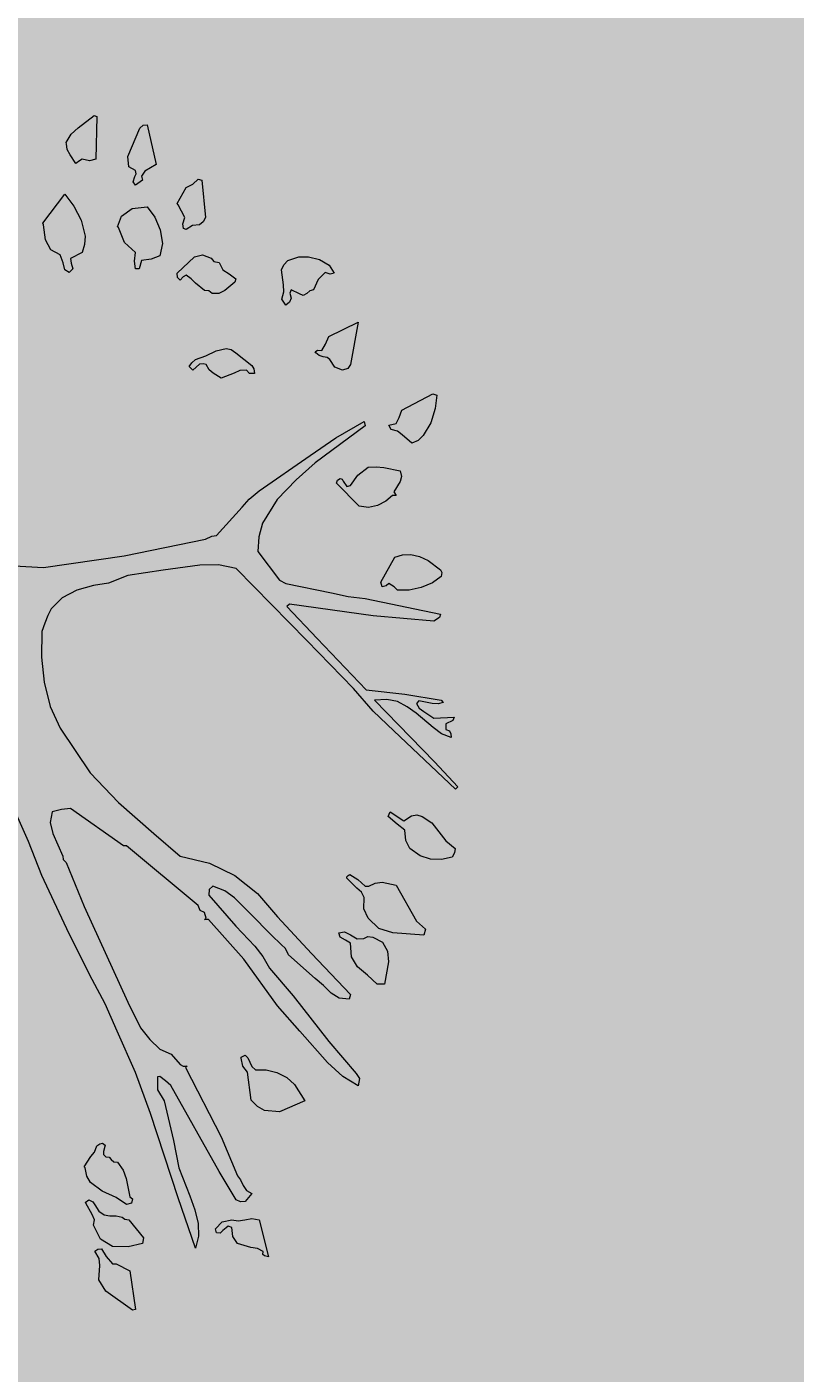
# Model space of a CAD drawing. Units: inches. Extents: x 84 to 1044, y -280 to 906.
# Tile 71 of 105: x 718.82 to 732.52, y 408.34 to 432.35. Entities that reach past the tile are written whole.
import ezdxf

# ---------------------------------------------------------------- set-up
doc = ezdxf.new("R2010")
doc.units = ezdxf.units.IN
doc.layers.add('A-ANNO-DIMS', color=2, linetype='Continuous', lineweight=18)
doc.layers.add('L-PLNT', color=114, linetype='Continuous', lineweight=15)
doc.layers.add('L-PLNT-PATT', color=9, linetype='Continuous', lineweight=9, true_color=0xafd9aa)
doc.styles.get("Standard").update_dxf_attribs({"font": 'arial.ttf'})
doc.dimstyles.get("Standard").update_dxf_attribs({"dimtxt": 0.18, "dimasz": 0.18, "dimexe": 0.18, "dimexo": 0.0625, "dimgap": 0.09, "dimtad": 0, "dimtih": 1, "dimtoh": 1, "dimdec": 4, "dimzin": 0, "dimdsep": 46, "dimtxsty": 'Standard', "dimcen": 0.09, "dimadec": 0, "dimazin": 0, "dimtfac": 1, "dimtdec": 4, "dimtofl": 0, "dimtmove": 0, "dimatfit": 3, "dimfxl": 1, "dimtolj": 1, "dimtzin": 0, "dimarcsym": 0})

# ---------------------------------------------------------------- blocks, each defined once
blk = doc.blocks.new('A$C37E508DF')
for p, q in [((0.9686, 1.4334), (0.9875, 1.4476)), ((0.9875, 1.4476), (0.9905, 1.4467)), ((0.9905, 1.4467), (0.9896, 1.3966)), ((0.9545, 1.4159), (0.9605, 1.4257)), ((0.9605, 1.4257), (0.9686, 1.4334)), ((1.0269, 1.3996), (1.0411, 1.433)), ((1.0411, 1.433), (1.045, 1.4365)), ((1.045, 1.4365), (1.0497, 1.4369)), ((1.0497, 1.4369), (1.0604, 1.3901)), ((0.9549, 1.4146), (0.9545, 1.4159)), ((0.9558, 1.4077), (0.9549, 1.4146)), ((0.9592, 1.4017), (0.9558, 1.4077)), ((0.966, 1.3914), (0.9592, 1.4017)), ((0.9703, 1.3944), (0.966, 1.3914)), ((0.9733, 1.3966), (0.9703, 1.3944)), ((0.9819, 1.3944), (0.9733, 1.3966)), ((0.9896, 1.3966), (0.9819, 1.3944)), ((1.0282, 1.3876), (1.0269, 1.3996)), ((1.0359, 1.3833), (1.0282, 1.3876)), ((1.0334, 1.37), (1.0351, 1.376)), ((1.0351, 1.376), (1.0368, 1.3794)), ((1.0368, 1.3794), (1.0359, 1.3833)), ((1.0471, 1.3824), (1.0432, 1.3764)), ((1.0432, 1.3764), (1.0441, 1.3717)), ((1.0604, 1.3901), (1.0471, 1.3824)), ((1.0359, 1.3661), (1.0334, 1.37)), ((1.0441, 1.3717), (1.0359, 1.3661)), ((1.0848, 1.3443), (1.0955, 1.3631)), ((1.0955, 1.3631), (1.1033, 1.367)), ((1.1033, 1.367), (1.1097, 1.373)), ((1.1097, 1.373), (1.114, 1.3717)), ((1.114, 1.3717), (1.1183, 1.328)), ((0.9274, 1.3215), (0.9532, 1.3554)), ((0.9532, 1.3554), (0.9635, 1.3413)), ((1.0861, 1.343), (1.0848, 1.3443)), ((0.9635, 1.3413), (0.9721, 1.325)), ((1.0171, 1.3232), (1.0197, 1.3297)), ((1.0197, 1.3297), (1.0321, 1.3387)), ((1.0321, 1.3387), (1.0497, 1.3404)), ((1.0497, 1.3404), (1.0587, 1.3284)), ((1.0587, 1.3284), (1.0651, 1.3134)), ((1.0938, 1.328), (1.0861, 1.343)), ((1.0917, 1.3207), (1.0938, 1.328)), ((1.1183, 1.328), (1.1153, 1.3228)), ((0.9279, 1.3194), (0.9274, 1.3215)), ((0.9305, 1.3018), (0.9279, 1.3194)), ((0.9721, 1.325), (0.9768, 1.3061)), ((1.0149, 1.3172), (1.0171, 1.3232)), ((1.0162, 1.3164), (1.0149, 1.3172)), ((1.0231, 1.2988), (1.0162, 1.3164)), ((1.0651, 1.3134), (1.0677, 1.2975)), ((1.0925, 1.3151), (1.0917, 1.3207)), ((1.0955, 1.3138), (1.0925, 1.3151)), ((1.1028, 1.3185), (1.0955, 1.3138)), ((1.111, 1.3194), (1.1028, 1.3185)), ((1.1153, 1.3228), (1.111, 1.3194)), ((0.9365, 1.2902), (0.9305, 1.3018)), ((0.9763, 1.2962), (0.9733, 1.2868)), ((0.9768, 1.3061), (0.9763, 1.2962)), ((1.0359, 1.2868), (1.0231, 1.2988)), ((1.0677, 1.2975), (1.0647, 1.2829)), ((0.9476, 1.2842), (0.9365, 1.2902)), ((0.951, 1.2748), (0.9476, 1.2842)), ((0.9733, 1.2868), (0.9596, 1.2799)), ((0.9596, 1.2799), (0.9605, 1.2744)), ((1.0347, 1.2769), (1.0359, 1.2868)), ((1.0647, 1.2829), (1.0544, 1.2791)), ((1.0848, 1.2628), (1.1054, 1.2817)), ((1.1054, 1.2817), (1.1148, 1.2842)), ((1.1148, 1.2842), (1.1247, 1.2804)), ((1.1247, 1.2804), (1.1281, 1.2765)), ((1.2147, 1.2774), (1.2276, 1.2817)), ((1.2276, 1.2817), (1.2392, 1.2817)), ((1.2392, 1.2817), (1.2521, 1.2787)), ((0.9532, 1.2666), (0.951, 1.2748)), ((0.9583, 1.2636), (0.9532, 1.2666)), ((0.9626, 1.2679), (0.9583, 1.2636)), ((0.9605, 1.2744), (0.9626, 1.2679)), ((1.0359, 1.2679), (1.0347, 1.2769)), ((1.0402, 1.2679), (1.0359, 1.2679)), ((1.0432, 1.2774), (1.0402, 1.2679)), ((1.0544, 1.2791), (1.0432, 1.2774)), ((1.1281, 1.2765), (1.1341, 1.2752)), ((1.1341, 1.2752), (1.1384, 1.2666)), ((1.1384, 1.2666), (1.1461, 1.2619)), ((1.2075, 1.2666), (1.21, 1.2726)), ((1.2096, 1.2491), (1.2075, 1.2666)), ((1.21, 1.2726), (1.2147, 1.2774)), ((1.2521, 1.2787), (1.2632, 1.2722)), ((1.2632, 1.2722), (1.2692, 1.2628)), ((1.0852, 1.2576), (1.0848, 1.2628)), ((1.0883, 1.2546), (1.0852, 1.2576)), ((1.0921, 1.2585), (1.0883, 1.2546)), ((1.0955, 1.2602), (1.0921, 1.2585)), ((1.1015, 1.2559), (1.0955, 1.2602)), ((1.1063, 1.2508), (1.1015, 1.2559)), ((1.117, 1.2422), (1.1063, 1.2508)), ((1.1526, 1.2521), (1.141, 1.2422)), ((1.1461, 1.2619), (1.1539, 1.2559)), ((1.1539, 1.2559), (1.1526, 1.2521)), ((1.21, 1.2409), (1.2096, 1.2491)), ((1.2503, 1.2551), (1.2448, 1.2431)), ((1.2585, 1.2636), (1.2503, 1.2551)), ((1.2645, 1.2615), (1.2585, 1.2636)), ((1.2692, 1.2628), (1.2645, 1.2615)), ((1.1221, 1.2418), (1.117, 1.2422)), ((1.126, 1.2388), (1.1221, 1.2418)), ((1.1337, 1.2388), (1.126, 1.2388)), ((1.141, 1.2422), (1.1337, 1.2388)), ((1.2079, 1.2323), (1.21, 1.2409)), ((1.2186, 1.2332), (1.2169, 1.2285)), ((1.2186, 1.2431), (1.2173, 1.2392)), ((1.2173, 1.2392), (1.2186, 1.2332)), ((1.2285, 1.2383), (1.2186, 1.2431)), ((1.2328, 1.2366), (1.2285, 1.2383)), ((1.2371, 1.2388), (1.2328, 1.2366)), ((1.2405, 1.2418), (1.2371, 1.2388)), ((1.2448, 1.2431), (1.2405, 1.2418)), ((1.2126, 1.2251), (1.2079, 1.2323)), ((1.2169, 1.2285), (1.2126, 1.2251)), ((1.2628, 1.1882), (1.2975, 1.2053)), ((1.2975, 1.2053), (1.2885, 1.1556)), ((1.2589, 1.1792), (1.2628, 1.1882)), ((1.1187, 1.1655), (1.1307, 1.1714)), ((1.1307, 1.1714), (1.1423, 1.1744)), ((1.1423, 1.1744), (1.1483, 1.1732)), ((1.1483, 1.1732), (1.1539, 1.1693)), ((1.1539, 1.1693), (1.1727, 1.1543)), ((1.2469, 1.1702), (1.2495, 1.1723)), ((1.2478, 1.1693), (1.2469, 1.1702)), ((1.2516, 1.1659), (1.2478, 1.1693)), ((1.2495, 1.1723), (1.2546, 1.1719)), ((1.2546, 1.1719), (1.2589, 1.1792)), ((1.099, 1.153), (1.102, 1.1573)), ((1.102, 1.1573), (1.1063, 1.1612)), ((1.111, 1.156), (1.1033, 1.1487)), ((1.1063, 1.1612), (1.1187, 1.1655)), ((1.1153, 1.1564), (1.111, 1.156)), ((1.1191, 1.1556), (1.1153, 1.1564)), ((1.1226, 1.1492), (1.1191, 1.1556)), ((1.1727, 1.1543), (1.1749, 1.1504)), ((1.2563, 1.1646), (1.2516, 1.1659)), ((1.2611, 1.1637), (1.2563, 1.1646)), ((1.2641, 1.1612), (1.2611, 1.1637)), ((1.2701, 1.1522), (1.2641, 1.1612)), ((1.2885, 1.1556), (1.2851, 1.1509)), ((1.1033, 1.1487), (1.099, 1.153)), ((1.1273, 1.1453), (1.1226, 1.1492)), ((1.1367, 1.1393), (1.1273, 1.1453)), ((1.1517, 1.1453), (1.1367, 1.1393)), ((1.1586, 1.1483), (1.1517, 1.1453)), ((1.1663, 1.1487), (1.1586, 1.1483)), ((1.1697, 1.1449), (1.1663, 1.1487)), ((1.1757, 1.1449), (1.1697, 1.1449)), ((1.1749, 1.1504), (1.1757, 1.1449)), ((1.2791, 1.1487), (1.2701, 1.1522)), ((1.2851, 1.1509), (1.2791, 1.1487)), ((1.3485, 1.102), (1.385, 1.1209)), ((1.385, 1.1209), (1.3897, 1.1196)), ((1.3897, 1.1196), (1.3875, 1.1037)), ((1.3421, 1.0861), (1.3455, 1.0934)), ((1.3455, 1.0934), (1.3485, 1.102)), ((1.3875, 1.1037), (1.3828, 1.087)), ((1.3057, 1.0835), (1.2469, 1.0402)), ((1.2713, 1.0694), (1.3044, 1.0887)), ((1.3044, 1.0887), (1.3057, 1.0835)), ((1.3335, 1.0844), (1.3421, 1.0861)), ((1.3361, 1.0793), (1.3335, 1.0844)), ((1.3434, 1.0771), (1.3361, 1.0793)), ((1.349, 1.0728), (1.3434, 1.0771)), ((1.3828, 1.087), (1.3738, 1.072)), ((1.2409, 1.0488), (1.2713, 1.0694)), ((1.3605, 1.063), (1.349, 1.0728)), ((1.3678, 1.0664), (1.3605, 1.063)), ((1.3738, 1.072), (1.3678, 1.0664)), ((1.1813, 1.0072), (1.2409, 1.0488)), ((1.2469, 1.0402), (1.2246, 1.0201)), ((1.2971, 1.0257), (1.3091, 1.0351)), ((1.3091, 1.0351), (1.3185, 1.0355)), ((1.3185, 1.0355), (1.3275, 1.0347)), ((1.3275, 1.0347), (1.3468, 1.0308)), ((1.3468, 1.0308), (1.3481, 1.0239)), ((1.2246, 1.0201), (1.2023, 0.9969)), ((1.2718, 1.0162), (1.2731, 1.0197)), ((1.2984, 0.9892), (1.2718, 1.0162)), ((1.2731, 1.0197), (1.2761, 1.0218)), ((1.2761, 1.0218), (1.2786, 1.0209)), ((1.2786, 1.0209), (1.2799, 1.0184)), ((1.2799, 1.0184), (1.2842, 1.0124)), ((1.2842, 1.0124), (1.2885, 1.0136)), ((1.2885, 1.0136), (1.2971, 1.0257)), ((1.3468, 1.018), (1.3391, 1.0059)), ((1.3481, 1.0239), (1.3468, 1.018)), ((1.1612, 0.9879), (1.1693, 0.9974)), ((1.1693, 0.9974), (1.1813, 1.0072)), ((1.2023, 0.9969), (1.1852, 0.9691)), ((1.3378, 1.0016), (1.3297, 0.9952)), ((1.3421, 1.0016), (1.3378, 1.0016)), ((1.3391, 1.0059), (1.3421, 1.0016)), ((1.1311, 0.9549), (1.1612, 0.9879)), ((1.3095, 0.9875), (1.2984, 0.9892)), ((1.3202, 0.9901), (1.3095, 0.9875)), ((1.3297, 0.9952), (1.3202, 0.9901)), ((1.1852, 0.9691), (1.1809, 0.9532)), ((1.0227, 0.9309), (1.1183, 0.9506)), ((1.1183, 0.9506), (1.1256, 0.954)), ((1.1256, 0.954), (1.1311, 0.9549)), ((1.1809, 0.9532), (1.1796, 0.936)), ((1.1796, 0.936), (1.2049, 0.9022)), ((1.3404, 0.9292), (1.3494, 0.9322)), ((1.3494, 0.9322), (1.3592, 0.9326)), ((1.3592, 0.9326), (1.3695, 0.93)), ((0.8936, 0.9193), (0.9279, 0.9172)), ((0.9279, 0.9172), (1.0227, 0.9309)), ((1.1114, 0.9198), (1.0685, 0.9142)), ((1.1333, 0.9202), (1.1114, 0.9198)), ((1.1543, 0.9159), (1.1333, 0.9202)), ((1.3241, 0.9), (1.3404, 0.9292)), ((1.3695, 0.93), (1.3794, 0.9253)), ((1.3794, 0.9253), (1.394, 0.9146)), ((1.0269, 0.9077), (1.0042, 0.8987)), ((1.0685, 0.9142), (1.0269, 0.9077)), ((1.2371, 0.8314), (1.1543, 0.9159)), ((1.2049, 0.9022), (1.2126, 0.8983)), ((1.3948, 0.9065), (1.3846, 0.8992)), ((1.394, 0.9146), (1.3957, 0.9112)), ((1.3957, 0.9112), (1.3948, 0.9065)), ((0.9673, 0.8906), (0.9498, 0.8816)), ((0.9866, 0.8962), (0.9673, 0.8906)), ((1.0042, 0.8987), (0.9866, 0.8962)), ((1.2126, 0.8983), (1.2662, 0.8876)), ((1.2662, 0.8876), (1.2855, 0.8833)), ((1.3254, 0.8944), (1.3241, 0.9)), ((1.3301, 0.8957), (1.3254, 0.8944)), ((1.3335, 0.8983), (1.3301, 0.8957)), ((1.3395, 0.8944), (1.3335, 0.8983)), ((1.3434, 0.8906), (1.3395, 0.8944)), ((1.3571, 0.8906), (1.3434, 0.8906)), ((1.3713, 0.8936), (1.3571, 0.8906)), ((1.3846, 0.8992), (1.3713, 0.8936)), ((0.9498, 0.8816), (0.9369, 0.8687)), ((1.2169, 0.8743), (1.2135, 0.8713)), ((1.2135, 0.8713), (1.2491, 0.834)), ((1.3151, 0.8606), (1.2169, 0.8743)), ((1.2855, 0.8833), (1.3057, 0.8807)), ((1.3057, 0.8807), (1.394, 0.8623)), ((0.933, 0.861), (0.9296, 0.852)), ((0.9369, 0.8687), (0.933, 0.861)), ((1.3863, 0.8541), (1.3151, 0.8606)), ((1.3927, 0.8584), (1.3863, 0.8541)), ((1.394, 0.8623), (1.3927, 0.8584)), ((0.9262, 0.8421), (0.9257, 0.8121)), ((0.9296, 0.852), (0.9262, 0.8421)), ((1.2919, 0.7752), (1.2371, 0.8314)), ((1.2491, 0.834), (1.3069, 0.7735)), ((0.9257, 0.8121), (0.9287, 0.7825)), ((0.9287, 0.7825), (0.936, 0.7542)), ((1.3151, 0.7487), (1.2919, 0.7752)), ((1.3069, 0.7735), (1.352, 0.7684)), ((1.3309, 0.7624), (1.3164, 0.7615)), ((1.3164, 0.7615), (1.3871, 0.6891)), ((1.3434, 0.7598), (1.3309, 0.7624)), ((1.355, 0.7538), (1.3434, 0.7598)), ((1.352, 0.7684), (1.3948, 0.7615)), ((1.3687, 0.7607), (1.3657, 0.7577)), ((1.3841, 0.7577), (1.3687, 0.7607)), ((1.397, 0.759), (1.3914, 0.7572)), ((1.3948, 0.7615), (1.397, 0.759)), ((0.936, 0.7542), (0.9476, 0.7285)), ((1.3391, 0.7255), (1.3151, 0.7487)), ((1.3653, 0.7461), (1.355, 0.7538)), ((1.3854, 0.7294), (1.3653, 0.7461)), ((1.3657, 0.7577), (1.3691, 0.7521)), ((1.3691, 0.7521), (1.3743, 0.7482)), ((1.3743, 0.7482), (1.3863, 0.7405)), ((1.3914, 0.7572), (1.3841, 0.7577)), ((0.9476, 0.7285), (0.9828, 0.6762)), ((1.3953, 0.7221), (1.3854, 0.7294)), ((1.3863, 0.7405), (1.4099, 0.7414)), ((1.4086, 0.7375), (1.4004, 0.7337)), ((1.4004, 0.7337), (1.4004, 0.7272)), ((1.4004, 0.7272), (1.4047, 0.7255)), ((1.4099, 0.7414), (1.4086, 0.7375)), ((1.4116, 0.6569), (1.3391, 0.7255)), ((1.4064, 0.7178), (1.3953, 0.7221)), ((1.4047, 0.7255), (1.406, 0.7221)), ((1.406, 0.7221), (1.4064, 0.7178)), ((1.3871, 0.6891), (1.4141, 0.6599)), ((0.9828, 0.6762), (1.0162, 0.6415)), ((1.4141, 0.6599), (1.4116, 0.6569)), ((0.9103, 0.5956), (0.8932, 0.6342)), ((0.9493, 0.6333), (0.9382, 0.6303)), ((0.9596, 0.6342), (0.9493, 0.6333)), ((1.0218, 0.5904), (0.9596, 0.6342)), ((1.0162, 0.6415), (1.0574, 0.605)), ((0.9382, 0.6303), (0.936, 0.6179)), ((0.936, 0.6179), (0.939, 0.605)), ((1.3327, 0.6252), (1.3348, 0.6303)), ((1.343, 0.6162), (1.3327, 0.6252)), ((1.3348, 0.6303), (1.3511, 0.62)), ((1.3511, 0.62), (1.3601, 0.6256)), ((1.3601, 0.6256), (1.3661, 0.6269)), ((1.3661, 0.6269), (1.3725, 0.6252)), ((1.3725, 0.6252), (1.3837, 0.6175)), ((1.3837, 0.6175), (1.3918, 0.6072)), ((0.939, 0.605), (0.9506, 0.5784)), ((1.0574, 0.605), (1.0883, 0.5784)), ((1.352, 0.6089), (1.343, 0.6162)), ((1.3533, 0.5969), (1.352, 0.6089)), ((1.3918, 0.6072), (1.4004, 0.5964)), ((0.9262, 0.5557), (0.9103, 0.5956)), ((1.0256, 0.5904), (1.0218, 0.5904)), ((1.1097, 0.5205), (1.0256, 0.5904)), ((1.358, 0.5874), (1.3533, 0.5969)), ((1.37, 0.5789), (1.358, 0.5874)), ((1.4004, 0.5964), (1.4111, 0.5874)), ((1.4111, 0.5874), (1.4103, 0.5823)), ((0.9506, 0.5784), (0.951, 0.5746)), ((0.951, 0.5746), (0.9545, 0.5711)), ((0.9545, 0.5711), (0.9759, 0.5193)), ((1.0883, 0.5784), (1.123, 0.5703)), ((1.123, 0.5703), (1.1526, 0.5557)), ((1.3824, 0.575), (1.37, 0.5789)), ((1.3953, 0.5746), (1.3824, 0.575)), ((1.4077, 0.5771), (1.3953, 0.5746)), ((1.4103, 0.5823), (1.4077, 0.5771)), ((0.9583, 0.4871), (0.9262, 0.5557)), ((1.1526, 0.5557), (1.1792, 0.5347)), ((1.2842, 0.554), (1.2855, 0.5557)), ((1.2842, 0.5527), (1.2842, 0.554)), ((1.2855, 0.5557), (1.2876, 0.557)), ((1.2876, 0.557), (1.2971, 0.551)), ((1.1226, 0.5394), (1.1221, 0.5325)), ((1.1268, 0.5433), (1.1226, 0.5394)), ((1.141, 0.5377), (1.1268, 0.5433)), ((1.1521, 0.5296), (1.141, 0.5377)), ((1.2958, 0.5407), (1.2842, 0.5527)), ((1.3014, 0.536), (1.2958, 0.5407)), ((1.2971, 0.551), (1.3057, 0.5433)), ((1.3057, 0.5433), (1.3099, 0.5433)), ((1.3099, 0.5433), (1.3172, 0.5467)), ((1.3172, 0.5467), (1.3254, 0.548)), ((1.3254, 0.548), (1.3421, 0.5446)), ((1.3421, 0.5446), (1.3657, 0.5021)), ((1.1221, 0.5325), (1.1539, 0.4961)), ((1.1706, 0.5111), (1.1521, 0.5296)), ((1.1792, 0.5347), (1.2027, 0.5072)), ((1.3044, 0.53), (1.3014, 0.536)), ((1.3039, 0.5167), (1.3044, 0.53)), ((0.9759, 0.5193), (1.0269, 0.4069)), ((1.1118, 0.5145), (1.1097, 0.5205)), ((1.117, 0.5124), (1.1118, 0.5145)), ((1.1191, 0.5055), (1.117, 0.5124)), ((1.1955, 0.4858), (1.1706, 0.5111)), ((1.2027, 0.5072), (1.2426, 0.4644)), ((1.3091, 0.5055), (1.3039, 0.5167)), ((1.117, 0.5042), (1.1191, 0.5055)), ((1.1217, 0.5042), (1.117, 0.5042)), ((1.1633, 0.4575), (1.1217, 0.5042)), ((1.1539, 0.4961), (1.1762, 0.4729)), ((1.3215, 0.4935), (1.3091, 0.5055)), ((1.3382, 0.4884), (1.3215, 0.4935)), ((1.3657, 0.5021), (1.3764, 0.4927)), ((1.3764, 0.4927), (1.3743, 0.4858)), ((0.9853, 0.4335), (0.9583, 0.4871)), ((1.207, 0.4747), (1.1955, 0.4858)), ((1.2122, 0.47), (1.207, 0.4747)), ((1.2748, 0.4884), (1.2812, 0.4897)), ((1.2761, 0.4832), (1.2748, 0.4884)), ((1.2825, 0.4798), (1.2761, 0.4832)), ((1.2812, 0.4897), (1.2885, 0.4862)), ((1.2885, 0.4764), (1.2825, 0.4798)), ((1.2885, 0.4862), (1.2962, 0.4815)), ((1.2894, 0.4601), (1.2885, 0.4764)), ((1.2962, 0.4815), (1.3039, 0.482)), ((1.3039, 0.482), (1.3087, 0.4841)), ((1.3087, 0.4841), (1.3147, 0.4832)), ((1.3147, 0.4832), (1.3258, 0.4777)), ((1.3258, 0.4777), (1.3318, 0.4669)), ((1.3743, 0.4858), (1.3382, 0.4884)), ((1.1762, 0.4729), (1.1856, 0.4605)), ((1.1856, 0.4605), (1.1933, 0.4468)), ((1.2156, 0.4627), (1.2122, 0.47)), ((1.2469, 0.4348), (1.2156, 0.4627)), ((1.2426, 0.4644), (1.2885, 0.4159)), ((1.2967, 0.4485), (1.2894, 0.4601)), ((1.3318, 0.4669), (1.3331, 0.4545)), ((1.2027, 0.4026), (1.1633, 0.4575)), ((1.1933, 0.4468), (1.2212, 0.4146)), ((1.3082, 0.4386), (1.2967, 0.4485)), ((1.3331, 0.4545), (1.3284, 0.4284)), ((1.0003, 0.4052), (0.9853, 0.4335)), ((1.2568, 0.4266), (1.2469, 0.4348)), ((1.2658, 0.4176), (1.2568, 0.4266)), ((1.3198, 0.4284), (1.3082, 0.4386)), ((1.3284, 0.4284), (1.3198, 0.4284)), ((1.2212, 0.4146), (1.2628, 0.361)), ((1.2752, 0.4116), (1.2658, 0.4176)), ((1.2868, 0.4108), (1.2752, 0.4116)), ((1.2885, 0.4159), (1.2868, 0.4108)), ((1.0145, 0.373), (1.0003, 0.4052)), ((1.0269, 0.4069), (1.0419, 0.3769)), ((1.2289, 0.373), (1.2027, 0.4026)), ((1.0359, 0.3246), (1.0145, 0.373)), ((1.0419, 0.3769), (1.0527, 0.3632)), ((1.2615, 0.3362), (1.2289, 0.373)), ((1.0527, 0.3632), (1.0647, 0.352)), ((1.0647, 0.352), (1.078, 0.346)), ((1.2628, 0.361), (1.2949, 0.3233)), ((1.078, 0.346), (1.0883, 0.334)), ((1.0883, 0.334), (1.0921, 0.3319)), ((1.0921, 0.3319), (1.0968, 0.3319)), ((1.0968, 0.3319), (1.0947, 0.3306)), ((1.1599, 0.3426), (1.1646, 0.3447)), ((1.1599, 0.3413), (1.1599, 0.3426)), ((1.162, 0.3319), (1.1599, 0.3413)), ((1.1676, 0.325), (1.162, 0.3319)), ((1.1646, 0.3447), (1.168, 0.3417)), ((1.168, 0.3417), (1.1702, 0.3366)), ((1.1702, 0.3366), (1.1727, 0.3314)), ((1.2795, 0.3199), (1.2615, 0.3362)), ((1.0535, 0.2766), (1.0359, 0.3246)), ((1.0647, 0.3199), (1.0617, 0.3194)), ((1.0617, 0.3194), (1.0617, 0.304)), ((1.0711, 0.3147), (1.0647, 0.3199)), ((1.0947, 0.3306), (1.1367, 0.2491)), ((1.1719, 0.292), (1.1676, 0.325)), ((1.1727, 0.3314), (1.177, 0.3276)), ((1.177, 0.3276), (1.1895, 0.3276)), ((1.1895, 0.3276), (1.2019, 0.3246)), ((1.2019, 0.3246), (1.2135, 0.3186)), ((1.2135, 0.3186), (1.2225, 0.3104)), ((1.2975, 0.3087), (1.2795, 0.3199)), ((1.2949, 0.3233), (1.2988, 0.3173)), ((1.2988, 0.3173), (1.2975, 0.3087)), ((1.0617, 0.304), (1.0698, 0.2911)), ((1.0775, 0.3092), (1.0711, 0.3147)), ((1.1341, 0.2084), (1.0775, 0.3092)), ((1.2225, 0.3104), (1.2349, 0.2911)), ((1.0698, 0.2911), (1.0805, 0.2448)), ((1.1792, 0.2847), (1.1719, 0.292)), ((1.1873, 0.28), (1.1792, 0.2847)), ((1.2349, 0.2911), (1.2049, 0.2783)), ((1.0861, 0.1775), (1.0535, 0.2766)), ((1.2049, 0.2783), (1.1873, 0.28)), ((0.9879, 0.2311), (0.9905, 0.2384)), ((0.9905, 0.2384), (0.9943, 0.241)), ((0.9943, 0.241), (0.9973, 0.2414)), ((0.9973, 0.2414), (1.0003, 0.2393)), ((1.0003, 0.2393), (0.9986, 0.232)), ((1.0805, 0.2448), (1.087, 0.2127)), ((1.1367, 0.2491), (1.1556, 0.2032)), ((0.9759, 0.214), (0.9836, 0.226)), ((0.9836, 0.226), (0.9879, 0.2311)), ((0.9986, 0.232), (0.9986, 0.2281)), ((0.9986, 0.2281), (1.0012, 0.2255)), ((1.0012, 0.2255), (1.0051, 0.2251)), ((1.0051, 0.2251), (1.0076, 0.2225)), ((1.0076, 0.2225), (1.0106, 0.2195)), ((0.9768, 0.2127), (0.9759, 0.214)), ((0.9789, 0.2028), (0.9768, 0.2127)), ((1.0106, 0.2195), (1.0149, 0.2191)), ((1.0149, 0.2191), (1.0214, 0.2101)), ((1.0214, 0.2101), (1.0252, 0.2002)), ((1.087, 0.2127), (1.0998, 0.1797)), ((1.1543, 0.1749), (1.1341, 0.2084)), ((0.9832, 0.1955), (0.9789, 0.2028)), ((0.9969, 0.1852), (0.9832, 0.1955)), ((1.0252, 0.2002), (1.0295, 0.1788)), ((1.1556, 0.2032), (1.1594, 0.1985)), ((1.1594, 0.1985), (1.1624, 0.1921)), ((1.1624, 0.1921), (1.1663, 0.1861)), ((0.9768, 0.1719), (0.9811, 0.1749)), ((0.9811, 0.1749), (0.9858, 0.1728)), ((1.0132, 0.1779), (0.9969, 0.1852)), ((1.0256, 0.1698), (1.0132, 0.1779)), ((1.0295, 0.1788), (1.0325, 0.1762)), ((1.0325, 0.1762), (1.0312, 0.1711)), ((1.1063, 0.1183), (1.0861, 0.1775)), ((1.0998, 0.1797), (1.1058, 0.1634)), ((1.1594, 0.1728), (1.1543, 0.1749)), ((1.1727, 0.1827), (1.1646, 0.1732)), ((1.1663, 0.1861), (1.1727, 0.1827)), ((0.9776, 0.1711), (0.9768, 0.1719)), ((0.9853, 0.1578), (0.9776, 0.1711)), ((0.9858, 0.1728), (0.9884, 0.1694)), ((0.9884, 0.1694), (0.9931, 0.1616)), ((0.9931, 0.1616), (0.9991, 0.1574)), ((1.0312, 0.1711), (1.0256, 0.1698)), ((1.1058, 0.1634), (1.1097, 0.1475)), ((1.1646, 0.1732), (1.1594, 0.1728)), ((0.9879, 0.1518), (0.9853, 0.1578)), ((0.9866, 0.1453), (0.9879, 0.1518)), ((0.9948, 0.1291), (0.9866, 0.1453)), ((0.9991, 0.1574), (1.0059, 0.1565)), ((1.0059, 0.1565), (1.0132, 0.1565)), ((1.0132, 0.1565), (1.0205, 0.1548)), ((1.0205, 0.1548), (1.0235, 0.1522)), ((1.0235, 0.1522), (1.0282, 0.1518)), ((1.0282, 0.1518), (1.0454, 0.1303)), ((1.1097, 0.1475), (1.1101, 0.1325)), ((1.1298, 0.1411), (1.1376, 0.1492)), ((1.1376, 0.1492), (1.1491, 0.1518)), ((1.1423, 0.1423), (1.1384, 0.1389)), ((1.1449, 0.1441), (1.1423, 0.1423)), ((1.1491, 0.1428), (1.1449, 0.1441)), ((1.1491, 0.1518), (1.1564, 0.1505)), ((1.1504, 0.132), (1.1491, 0.1428)), ((1.1564, 0.1505), (1.1642, 0.1518)), ((1.1642, 0.1518), (1.1727, 0.1531)), ((1.1727, 0.1531), (1.1813, 0.1518)), ((1.1813, 0.1518), (1.192, 0.108)), ((1.0089, 0.1205), (0.9948, 0.1291)), ((1.0454, 0.1303), (1.0441, 0.1239)), ((1.1101, 0.1325), (1.1063, 0.1183)), ((1.1311, 0.1364), (1.1298, 0.1411)), ((1.1354, 0.1359), (1.1311, 0.1364)), ((1.1384, 0.1389), (1.1354, 0.1359)), ((1.1556, 0.1239), (1.1504, 0.132)), ((0.9884, 0.1149), (0.9918, 0.117)), ((0.9935, 0.1063), (0.9884, 0.1149)), ((0.9918, 0.117), (0.9961, 0.1175)), ((0.9961, 0.1175), (1.0016, 0.1085)), ((1.0274, 0.12), (1.0089, 0.1205)), ((1.0441, 0.1239), (1.0274, 0.12)), ((1.1714, 0.1192), (1.1556, 0.1239)), ((1.1792, 0.1179), (1.1714, 0.1192)), ((1.186, 0.1145), (1.1792, 0.1179)), ((1.1856, 0.111), (1.186, 0.1145)), ((1.1873, 0.1093), (1.1856, 0.111)), ((0.9931, 0.081), (0.9943, 0.0982)), ((0.9943, 0.0982), (0.9935, 0.1063)), ((1.0016, 0.1085), (1.0089, 0.0999)), ((1.0089, 0.0999), (1.0132, 0.0999)), ((1.0132, 0.0999), (1.0295, 0.0917)), ((1.192, 0.108), (1.1873, 0.1093)), ((1.0012, 0.0677), (0.9931, 0.081)), ((1.0295, 0.0917), (1.0359, 0.0463)), ((1.0325, 0.0454), (1.0012, 0.0677)), ((1.0359, 0.0463), (1.0325, 0.0454))]:
    blk.add_line(p, q)
blk = doc.blocks.new('*D62')
at = {"layer": 'A-ANNO-DIMS', "color": 0, "lineweight": -2, "transparency": 16777216}
for p, q in [((203.179, 709.183), (203.179, 905.9)), ((896.074, 400.183), (896.074, 905.9)), ((203.359, 905.72), (549.232, 905.72)), ((895.894, 905.72), (550.021, 905.72))]:
    blk.add_line(p, q, dxfattribs=at)
at = {"layer": 'A-ANNO-DIMS', "color": 0, "transparency": 16777216}
for points in [[(203.359, 905.75), (203.359, 905.69), (203.179, 905.72)], [(895.894, 905.75), (895.894, 905.69), (896.074, 905.72)]]:
    blk.add_solid(points, dxfattribs=at)
at = {"layer": 'Defpoints', "color": 0, "transparency": 16777216}
for p in [(896.074, 905.72), (203.179, 709.12), (896.074, 400.12)]:
    blk.add_point(p, dxfattribs=at)
at = {"layer": 'A-ANNO-DIMS', "color": 0, "transparency": 16777216, "insert": (549.627, 905.72), "char_height": 0.18, "attachment_point": 5}
blk.add_mtext('\\A1;692.9', dxfattribs=at)

msp = doc.modelspace()

# ---------------------------------------------------------------- hatches: boundary and pattern name
at = {"layer": 'L-PLNT-PATT', "transparency": 33554597}
h = msp.add_hatch(color=256, dxfattribs=at)
h.dxf.hatch_style = 1
h.paths.add_polyline_path([(896.074, 511.12), (704.074, 511.12), (704.074, 491.62), (704.074, 419.62), (704.074, 400.12), (833.074, 400.12), (896.074, 400.12)])

# ---------------------------------------------------------------- block references
at = {"layer": 'L-PLNT', "xscale": 15.19586232982809, "yscale": 15.19586232982809, "zscale": 15.19586232982809}
msp.add_blockref('A$C37E508DF', (705.011, 408.771), dxfattribs=at)

# ---------------------------------------------------------------- dimensions: what is measured, and where the dimension line sits
at = {"layer": 'A-ANNO-DIMS'}
dim = msp.add_linear_dim(base=(896.074, 905.72), p1=(203.179, 709.12), p2=(896.074, 400.12), dimstyle='Standard', override={"dimdec": 1, "dimlfac": 1, "dimrnd": 0, "dimzin": 0, "dimdsep": 46, "dimlunit": 2}, dxfattribs=at)
dim.commit()
dim.dimension.update_dxf_attribs({"geometry": '*D62', "text_midpoint": (549.627, 905.72)})

doc.saveas('drawing.dxf')
